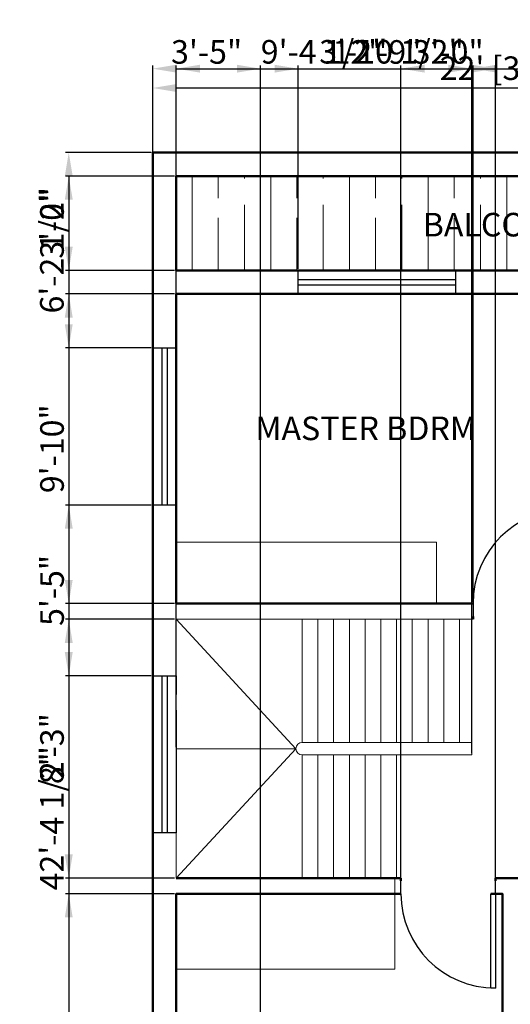
# Model space of a CAD drawing. Units: inches. Extents: x 2429 to 3343, y 1496 to 2530.
# Tile 6 of 7: x 2954 to 3141, y 2154 to 2529. Entities that reach past the tile are written whole.
import ezdxf

# ---------------------------------------------------------------- set-up
doc = ezdxf.new("R2010")
doc.units = ezdxf.units.IN
for name, color, linetype, lineweight in [('A-ANNO-DIMS', 2, 'Continuous', 18), ('A-AREA-IDEN', 3, 'Continuous', 18), ('A-DOOR', 3, 'Continuous', 25), ('A-FLOR-PATT', 8, 'Continuous', 13), ('A-FLOR-STRS', 2, 'Continuous', 18), ('A-FURN', 9, 'Continuous', 18), ('A-GLAZ', 4, 'Continuous', 25), ('A-WALL', 7, 'Continuous', 50)]:
    doc.layers.add(name, color=color, linetype=linetype, lineweight=lineweight)
doc.styles.get("Standard").update_dxf_attribs({"font": 'arial.ttf'})
doc.dimstyles.new('ISO-25', dxfattribs={"dimtxt": 9, "dimasz": 9, "dimexe": 1.25, "dimexo": 0.625, "dimtad": 1, "dimdec": 1, "dimlunit": 3, "dimtxsty": 'Standard', "dimcen": 9, "dimadec": 0, "dimazin": 0, "dimtfac": 1, "dimtdec": 1, "dimtmove": 0, "dimatfit": 3, "dimfxl": 1, "dimarcsym": 0})

# ---------------------------------------------------------------- blocks, each defined once
blk = doc.blocks.new('*D9')
at = {"layer": 'A-ANNO-DIMS', "color": 0, "lineweight": -2, "transparency": 16777216}
for p, q in [((3005.05, 2479.42), (3005.05, 2504.67)), ((3269.05, 2479.42), (3269.05, 2504.67)), ((3014.05, 2503.42), (3260.05, 2503.42))]:
    blk.add_line(p, q, dxfattribs=at)
at = {"layer": 'A-ANNO-DIMS', "color": 0, "transparency": 16777216}
for points in [[(3014.05, 2504.92), (3014.05, 2501.92), (3005.05, 2503.42)], [(3260.05, 2504.92), (3260.05, 2501.92), (3269.05, 2503.42)]]:
    blk.add_solid(points, dxfattribs=at)
at = {"layer": 'Defpoints', "color": 0, "transparency": 16777216}
for p in [(3269.05, 2503.42), (3005.05, 2478.79), (3269.05, 2478.79)]:
    blk.add_point(p, dxfattribs=at)
at = {"layer": 'A-ANNO-DIMS', "color": 0, "transparency": 16777216, "insert": (3137.05, 2509.81), "char_height": 9, "attachment_point": 5}
blk.add_mtext("22' [33']", dxfattribs=at)
blk = doc.blocks.new('*U2')
for p, q in [((0, 0), (0, -5)), ((-36, 0), (-36, -5))]:
    blk.add_line(p, q)
blk.add_lwpolyline([(0, 0), (0, 36), (-1.75, 36), (-1.75, 0)], close=True)
blk.add_arc((0, 0), 36, 90, 180)
blk = doc.blocks.new('*U12')
for p, q in [((-36, 0), (-36, 5)), ((0, 0), (0, 5))]:
    blk.add_line(p, q)
blk.add_lwpolyline([(0, 0), (0, -36), (-1.75, -36), (-1.75, 0)], close=True)
blk.add_arc((0, 0), 36, 180, 270)
blk = doc.blocks.new('WIN-PLAN-1500')
for p, q in [((3.5, 60), (3.5, 0)), ((5.5, 60), (5.5, 0))]:
    blk.add_line(p, q)
blk.add_lwpolyline([(9, 60), (9, 0), (0, 0), (0, 60)], close=True)
blk = doc.blocks.new('*D56')
at = {"layer": 'A-ANNO-DIMS', "color": 0, "lineweight": -2, "transparency": 16777216}
for p, q in [((3004.42, 2478.79), (2971.8, 2478.79)), ((2973.05, 2469.79), (2973.05, 1979.47)), ((3134.79, 1970.47), (2971.8, 1970.47))]:
    blk.add_line(p, q, dxfattribs=at)
at = {"layer": 'A-ANNO-DIMS', "color": 0, "transparency": 16777216}
for points in [[(2971.55, 2469.79), (2974.55, 2469.79), (2973.05, 2478.79)], [(2971.55, 1979.47), (2974.55, 1979.47), (2973.05, 1970.47)]]:
    blk.add_solid(points, dxfattribs=at)
at = {"layer": 'Defpoints', "color": 0, "transparency": 16777216}
for p in [(3005.05, 2478.79), (2973.05, 1970.47), (3135.41, 1970.47)]:
    blk.add_point(p, dxfattribs=at)
at = {"layer": 'A-ANNO-DIMS', "color": 0, "transparency": 16777216, "insert": (2967.77, 2224.63), "char_height": 9, "attachment_point": 5, "rotation": 90}
blk.add_mtext('42\'-4 1/2"', dxfattribs=at)
blk = doc.blocks.new('*D57')
at = {"layer": 'A-ANNO-DIMS', "color": 0, "lineweight": -2, "transparency": 16777216}
for p, q in [((3013.42, 2469.79), (2971.8, 2469.79)), ((2973.05, 2460.79), (2973.05, 2442.79)), ((3013.42, 2433.79), (2971.8, 2433.79))]:
    blk.add_line(p, q, dxfattribs=at)
at = {"layer": 'A-ANNO-DIMS', "color": 0, "transparency": 16777216}
for points in [[(2971.55, 2460.79), (2974.55, 2460.79), (2973.05, 2469.79)], [(2971.55, 2442.79), (2974.55, 2442.79), (2973.05, 2433.79)]]:
    blk.add_solid(points, dxfattribs=at)
at = {"layer": 'Defpoints', "color": 0, "transparency": 16777216}
for p in [(3014.05, 2469.79), (2973.05, 2433.79), (3014.05, 2433.79)]:
    blk.add_point(p, dxfattribs=at)
at = {"layer": 'A-ANNO-DIMS', "color": 0, "transparency": 16777216, "insert": (2967.83, 2451.79), "char_height": 9, "attachment_point": 5, "rotation": 90}
blk.add_mtext('3\'-0"', dxfattribs=at)
blk = doc.blocks.new('*D58')
at = {"layer": 'A-ANNO-DIMS', "color": 0, "lineweight": -2, "transparency": 16777216}
for p, q in [((3014.05, 2425.42), (3014.05, 2512.04)), ((3167.05, 2425.42), (3167.05, 2512.04)), ((3023.05, 2510.79), (3158.05, 2510.79))]:
    blk.add_line(p, q, dxfattribs=at)
at = {"layer": 'A-ANNO-DIMS', "color": 0, "transparency": 16777216}
for points in [[(3023.05, 2512.29), (3023.05, 2509.29), (3014.05, 2510.79)], [(3158.05, 2512.29), (3158.05, 2509.29), (3167.05, 2510.79)]]:
    blk.add_solid(points, dxfattribs=at)
at = {"layer": 'Defpoints', "color": 0, "transparency": 16777216}
for p in [(3167.05, 2510.79), (3014.05, 2424.79), (3167.05, 2424.79)]:
    blk.add_point(p, dxfattribs=at)
at = {"layer": 'A-ANNO-DIMS', "color": 0, "transparency": 16777216, "insert": (3090.55, 2516.01), "char_height": 9, "attachment_point": 5}
blk.add_mtext('12\'-9"', dxfattribs=at)
blk = doc.blocks.new('*D59')
at = {"layer": 'A-ANNO-DIMS', "color": 0, "lineweight": -2, "transparency": 16777216}
for p, q in [((3013.42, 2424.79), (2971.8, 2424.79)), ((2973.05, 2415.79), (2973.05, 2315.58)), ((3013.42, 2306.58), (2971.8, 2306.58))]:
    blk.add_line(p, q, dxfattribs=at)
at = {"layer": 'A-ANNO-DIMS', "color": 0, "transparency": 16777216}
for points in [[(2971.55, 2415.79), (2974.55, 2415.79), (2973.05, 2424.79)], [(2971.55, 2315.58), (2974.55, 2315.58), (2973.05, 2306.58)]]:
    blk.add_solid(points, dxfattribs=at)
at = {"layer": 'Defpoints', "color": 0, "transparency": 16777216}
for p in [(3014.05, 2424.79), (2973.05, 2306.58), (3014.05, 2306.58)]:
    blk.add_point(p, dxfattribs=at)
at = {"layer": 'A-ANNO-DIMS', "color": 0, "transparency": 16777216, "insert": (2967.83, 2365.69), "char_height": 9, "attachment_point": 5, "rotation": 90}
blk.add_mtext('9\'-10"', dxfattribs=at)
blk = doc.blocks.new('*D63')
at = {"layer": 'A-ANNO-DIMS', "color": 0, "lineweight": -2, "transparency": 16777216}
for p, q in [((3013.42, 2300.58), (2971.8, 2300.58)), ((2973.05, 2291.58), (2973.05, 2210.79)), ((3013.42, 2201.79), (2971.8, 2201.79))]:
    blk.add_line(p, q, dxfattribs=at)
at = {"layer": 'A-ANNO-DIMS', "color": 0, "transparency": 16777216}
for points in [[(2971.55, 2291.58), (2974.55, 2291.58), (2973.05, 2300.58)], [(2971.55, 2210.79), (2974.55, 2210.79), (2973.05, 2201.79)]]:
    blk.add_solid(points, dxfattribs=at)
at = {"layer": 'Defpoints', "color": 0, "transparency": 16777216}
for p in [(3014.05, 2300.58), (2973.05, 2201.79), (3014.05, 2201.79)]:
    blk.add_point(p, dxfattribs=at)
at = {"layer": 'A-ANNO-DIMS', "color": 0, "transparency": 16777216, "insert": (2967.83, 2251.18), "char_height": 9, "attachment_point": 5, "rotation": 90}
blk.add_mtext('8\'-3"', dxfattribs=at)
blk = doc.blocks.new('*D64')
at = {"layer": 'A-ANNO-DIMS', "color": 0, "lineweight": -2, "transparency": 16777216}
for p, q in [((3014.05, 2251.81), (3014.05, 2512.04)), ((3126.78, 2249.41), (3126.78, 2512.04)), ((3023.05, 2510.79), (3117.78, 2510.79))]:
    blk.add_line(p, q, dxfattribs=at)
at = {"layer": 'A-ANNO-DIMS', "color": 0, "transparency": 16777216}
for points in [[(3023.05, 2512.29), (3023.05, 2509.29), (3014.05, 2510.79)], [(3117.78, 2512.29), (3117.78, 2509.29), (3126.78, 2510.79)]]:
    blk.add_solid(points, dxfattribs=at)
at = {"layer": 'Defpoints', "color": 0, "transparency": 16777216}
for p in [(3126.78, 2510.79), (3014.05, 2251.18), (3126.78, 2248.78)]:
    blk.add_point(p, dxfattribs=at)
at = {"layer": 'A-ANNO-DIMS', "color": 0, "transparency": 16777216, "insert": (3070.41, 2516.07), "char_height": 9, "attachment_point": 5}
blk.add_mtext('9\'-4 1/2"', dxfattribs=at)
blk = doc.blocks.new('*D66')
at = {"layer": 'A-ANNO-DIMS', "color": 0, "lineweight": -2, "transparency": 16777216}
for p, q in [((3013.42, 2195.79), (2971.8, 2195.79)), ((2973.05, 2186.79), (2973.05, 2036.79)), ((3013.42, 2027.79), (2971.8, 2027.79))]:
    blk.add_line(p, q, dxfattribs=at)
at = {"layer": 'A-ANNO-DIMS', "color": 0, "transparency": 16777216}
for points in [[(2971.55, 2186.79), (2974.55, 2186.79), (2973.05, 2195.79)], [(2971.55, 2036.79), (2974.55, 2036.79), (2973.05, 2027.79)]]:
    blk.add_solid(points, dxfattribs=at)
at = {"layer": 'Defpoints', "color": 0, "transparency": 16777216}
for p in [(3014.05, 2195.79), (2973.05, 2027.79), (3014.05, 2027.79)]:
    blk.add_point(p, dxfattribs=at)
at = {"layer": 'A-ANNO-DIMS', "color": 0, "transparency": 16777216, "insert": (2967.83, 2111.79), "char_height": 9, "attachment_point": 5, "rotation": 90}
blk.add_mtext('14\'-0"', dxfattribs=at)
blk = doc.blocks.new('*D71')
at = {"layer": 'A-ANNO-DIMS', "color": 0, "lineweight": -2, "transparency": 16777216}
for p, q in [((3014.05, 2434.42), (3014.05, 2512.04)), ((3060.55, 2434.42), (3060.55, 2512.04)), ((3023.05, 2510.79), (3051.55, 2510.79)), ((3060.55, 2510.79), (3122.68, 2510.79))]:
    blk.add_line(p, q, dxfattribs=at)
at = {"layer": 'A-ANNO-DIMS', "color": 0, "transparency": 16777216}
for points in [[(3023.05, 2512.29), (3023.05, 2509.29), (3014.05, 2510.79)], [(3051.55, 2512.29), (3051.55, 2509.29), (3060.55, 2510.79)]]:
    blk.add_solid(points, dxfattribs=at)
at = {"layer": 'Defpoints', "color": 0, "transparency": 16777216}
for p in [(3060.55, 2510.79), (3014.05, 2433.79), (3060.55, 2433.79)]:
    blk.add_point(p, dxfattribs=at)
at = {"layer": 'A-ANNO-DIMS', "color": 0, "transparency": 16777216, "insert": (3096.11, 2516.07), "char_height": 9, "attachment_point": 5}
blk.add_mtext('3\'-10 1/2"', dxfattribs=at)
blk = doc.blocks.new('*D72')
at = {"layer": 'A-ANNO-DIMS', "color": 0, "lineweight": -2, "transparency": 16777216}
for p, q in [((3004.42, 2478.79), (2971.8, 2478.79)), ((2973.05, 2469.79), (2973.05, 2413.19)), ((3004.42, 2404.19), (2971.8, 2404.19))]:
    blk.add_line(p, q, dxfattribs=at)
at = {"layer": 'A-ANNO-DIMS', "color": 0, "transparency": 16777216}
for points in [[(2971.55, 2469.79), (2974.55, 2469.79), (2973.05, 2478.79)], [(2971.55, 2413.19), (2974.55, 2413.19), (2973.05, 2404.19)]]:
    blk.add_solid(points, dxfattribs=at)
at = {"layer": 'Defpoints', "color": 0, "transparency": 16777216}
for p in [(3005.05, 2478.79), (2973.05, 2404.19), (3005.05, 2404.19)]:
    blk.add_point(p, dxfattribs=at)
at = {"layer": 'A-ANNO-DIMS', "color": 0, "transparency": 16777216, "insert": (2967.77, 2441.49), "char_height": 9, "attachment_point": 5, "rotation": 90}
blk.add_mtext('6\'-2 1/2"', dxfattribs=at)
blk = doc.blocks.new('*D73')
at = {"layer": 'A-ANNO-DIMS', "color": 0, "lineweight": -2, "transparency": 16777216}
for p, q in [((3004.42, 2344.19), (2971.8, 2344.19)), ((2973.05, 2335.19), (2973.05, 2288.03)), ((3004.42, 2279.03), (2971.8, 2279.03))]:
    blk.add_line(p, q, dxfattribs=at)
at = {"layer": 'A-ANNO-DIMS', "color": 0, "transparency": 16777216}
for points in [[(2971.55, 2335.19), (2974.55, 2335.19), (2973.05, 2344.19)], [(2971.55, 2288.03), (2974.55, 2288.03), (2973.05, 2279.03)]]:
    blk.add_solid(points, dxfattribs=at)
at = {"layer": 'Defpoints', "color": 0, "transparency": 16777216}
for p in [(3005.05, 2344.19), (2973.05, 2279.03), (3005.05, 2279.03)]:
    blk.add_point(p, dxfattribs=at)
at = {"layer": 'A-ANNO-DIMS', "color": 0, "transparency": 16777216, "insert": (2967.85, 2311.61), "char_height": 9, "attachment_point": 5, "rotation": 90}
blk.add_mtext('5\'-5"', dxfattribs=at)
blk = doc.blocks.new('*D76')
at = {"layer": 'A-ANNO-DIMS', "color": 0, "lineweight": -2, "transparency": 16777216}
for p, q in [((3005.05, 2019.41), (3005.05, 2512.04)), ((3046.2, 2019.41), (3046.2, 2512.04)), ((3014.05, 2510.79), (3037.2, 2510.79))]:
    blk.add_line(p, q, dxfattribs=at)
at = {"layer": 'A-ANNO-DIMS', "color": 0, "transparency": 16777216}
for points in [[(3014.05, 2512.29), (3014.05, 2509.29), (3005.05, 2510.79)], [(3037.2, 2512.29), (3037.2, 2509.29), (3046.2, 2510.79)]]:
    blk.add_solid(points, dxfattribs=at)
at = {"layer": 'Defpoints', "color": 0, "transparency": 16777216}
for p in [(3046.2, 2510.79), (3005.05, 2018.79), (3046.2, 2018.79)]:
    blk.add_point(p, dxfattribs=at)
at = {"layer": 'A-ANNO-DIMS', "color": 0, "transparency": 16777216, "insert": (3025.62, 2516.02), "char_height": 9, "attachment_point": 5}
blk.add_mtext('3\'-5"', dxfattribs=at)
blk = doc.blocks.new('*D79')
at = {"layer": 'A-ANNO-DIMS', "color": 0, "lineweight": -2, "transparency": 16777216}
for p, q in [((3127.2, 2307.21), (3127.2, 2512.04)), ((3161.45, 2307.21), (3161.45, 2512.04)), ((3136.2, 2510.79), (3152.45, 2510.79)), ((3161.45, 2510.79), (3223.74, 2510.79))]:
    blk.add_line(p, q, dxfattribs=at)
at = {"layer": 'A-ANNO-DIMS', "color": 0, "transparency": 16777216}
for points in [[(3136.2, 2512.29), (3136.2, 2509.29), (3127.2, 2510.79)], [(3152.45, 2512.29), (3152.45, 2509.29), (3161.45, 2510.79)]]:
    blk.add_solid(points, dxfattribs=at)
at = {"layer": 'Defpoints', "color": 0, "transparency": 16777216}
for p in [(3161.45, 2510.79), (3127.2, 2306.58), (3161.45, 2306.58)]:
    blk.add_point(p, dxfattribs=at)
at = {"layer": 'A-ANNO-DIMS', "color": 0, "transparency": 16777216, "insert": (3197.09, 2516.07), "char_height": 9, "attachment_point": 5}
blk.add_mtext('2\'-10 1/2"', dxfattribs=at)
blk = doc.blocks.new('*D81')
at = {"layer": 'A-ANNO-DIMS', "color": 0, "lineweight": -2, "transparency": 16777216}
for p, q in [((3099.72, 2196.41), (3099.72, 2512.04)), ((3135.72, 2196.41), (3135.72, 2512.04)), ((3108.72, 2510.79), (3126.72, 2510.79))]:
    blk.add_line(p, q, dxfattribs=at)
at = {"layer": 'A-ANNO-DIMS', "color": 0, "transparency": 16777216}
for points in [[(3108.72, 2512.29), (3108.72, 2509.29), (3099.72, 2510.79)], [(3126.72, 2512.29), (3126.72, 2509.29), (3135.72, 2510.79)]]:
    blk.add_solid(points, dxfattribs=at)
at = {"layer": 'Defpoints', "color": 0, "transparency": 16777216}
for p in [(3135.72, 2510.79), (3099.72, 2195.79), (3135.72, 2195.79)]:
    blk.add_point(p, dxfattribs=at)
at = {"layer": 'A-ANNO-DIMS', "color": 0, "transparency": 16777216, "insert": (3117.72, 2516.02), "char_height": 9, "attachment_point": 5}
blk.add_mtext('3\'-0"', dxfattribs=at)

msp = doc.modelspace()

# ---------------------------------------------------------------- hatches: boundary and pattern name
at = {"layer": 'A-FLOR-PATT'}
h = msp.add_hatch(dxfattribs=at)
h.set_pattern_fill('GOST_WOOD', color=256, scale=5)
h.set_pattern_definition([(90, (3260.048, 2433.792), (30, -2e-15), [50, -10]), (90, (3270.048, 2423.792), (30, -2e-15), [30, -7.5, 15, -7.5]), (90, (3280.048, 2408.792), (30, -2e-15), [50, -10])])
h.paths.add_polyline_path([(3260.04839, 2469.7918), (3014.04839, 2469.7918), (3014.04839, 2433.7918), (3260.04839, 2433.7918)])
h.paths.add_polyline_path([(3104.56895, 2440.5916), (3163.9551, 2440.5916), (3163.9551, 2462.39929), (3104.56895, 2462.39929)], flags=24)

# ---------------------------------------------------------------- linework, layer by layer
at = {"layer": 'A-FLOR-STRS'}
for p, q in [((3014.04839, 2300.58253), (3127.19704, 2300.58253)), ((3062.04839, 2300.58253), (3062.04839, 2253.58451)), ((3068.04839, 2300.58253), (3068.04839, 2253.58451)), ((3074.04839, 2300.58253), (3074.04839, 2253.58451)), ((3080.04839, 2300.58253), (3080.04839, 2253.58451)), ((3086.04839, 2300.58253), (3086.04839, 2253.58451)), ((3092.04839, 2300.58253), (3092.04839, 2253.58451)), ((3098.04839, 2300.58253), (3098.04839, 2253.58451)), ((3104.04839, 2300.58253), (3104.04839, 2253.58451)), ((3110.04839, 2300.58253), (3110.04839, 2253.58451)), ((3116.04839, 2300.58253), (3116.04839, 2253.58451)), ((3122.04839, 2300.58253), (3122.04839, 2253.58451)), ((3059.64839, 2251.18451), (3014.04839, 2251.18451)), ((3068.04839, 2248.78451), (3068.04839, 2201.78649)), ((3074.04839, 2248.78451), (3074.04839, 2201.78649)), ((3080.04839, 2248.78451), (3080.04839, 2201.78649)), ((3086.04839, 2248.78451), (3086.04839, 2201.78649)), ((3092.04839, 2248.78451), (3092.04839, 2201.78649)), ((3098.04839, 2248.78451), (3098.04839, 2201.78649))]:
    msp.add_line(p, q, dxfattribs=at)
msp.add_lwpolyline([(3014.04839, 2300.58253), (3059.64839, 2251.18451), (3014.04839, 2201.78649)], close=True, dxfattribs=at)
msp.add_lwpolyline([(3126.78141, 2253.58451), (3126.78141, 2248.78451), (3062.04839, 2248.78451, -1), (3062.04839, 2253.58451)], format="xyb", close=True, dxfattribs=at)
msp.add_lwpolyline([(3062.04839, 2248.78451), (3062.04839, 2246.78451), (3062.04839, 2201.78649)], dxfattribs=at)
at = {"layer": 'A-FURN'}
for points in [[(3014.04839, 2329.96827), (3113.28676, 2329.96827), (3113.28676, 2306.58253)], [(3014.04839, 2167.02265), (3097.44138, 2167.02265), (3097.44138, 2201.78649)]]:
    msp.add_lwpolyline(points, dxfattribs=at)
at = {"layer": 'A-GLAZ'}
for p, q in [((3008.54839, 2279.02781), (3008.54839, 2219.02781)), ((3010.54839, 2279.02781), (3010.54839, 2219.02781))]:
    msp.add_line(p, q, dxfattribs=at)
msp.add_lwpolyline([(3014.04839, 2265.82385), (3014.04839, 2219.02781), (3005.04839, 2219.02781), (3005.04839, 2279.02781), (3014.04839, 2279.02781), (3014.04839, 2271.82385)], dxfattribs=at)
at = {"layer": 'A-WALL'}
for p, q in [((3127.19704, 2301.58253), (3127.19704, 2300.58253)), ((3099.7165, 2200.78649), (3099.7165, 2201.78649)), ((3135.7165, 2200.78649), (3135.7165, 2201.78649))]:
    msp.add_line(p, q, dxfattribs=at)
for points in [[(3135.41055, 1970.47184), (3269.04839, 1970.47184), (3269.04839, 2001.78649), (3269.04839, 2325.78649), (3269.04839, 2478.7918), (3005.04839, 2478.7918), (3005.04839, 2325.78649), (3005.04839, 2319.78649), (3005.04839, 2199.78649), (3005.04839, 2018.78649), (3135.41055, 2018.78649)], [(3260.04839, 2469.7918), (3014.04839, 2469.7918), (3014.04839, 2433.7918), (3260.04839, 2433.7918)]]:
    msp.add_lwpolyline(points, close=True, dxfattribs=at)
for points in [[(3127.19704, 2306.58253), (3014.04839, 2306.58253), (3014.04839, 2319.78649), (3014.04839, 2325.78649), (3014.04839, 2424.7918), (3167.04839, 2424.7918), (3167.04839, 2420.74151)], [(3099.7165, 2201.78649), (3014.04839, 2201.78649)], [(3149.96707, 2201.78649), (3135.7165, 2201.78649)], [(3133.9665, 2195.78649), (3138.41055, 2195.78649), (3138.41055, 2027.78649), (3014.04839, 2027.78649), (3014.04839, 2195.78649), (3099.7165, 2195.78649)]]:
    msp.add_lwpolyline(points, dxfattribs=at)

# ---------------------------------------------------------------- block references
at = {"layer": 'A-DOOR'}
for name, p in [('*U2', (3163.19704, 2306.58253)), ('*U12', (3135.7165, 2195.78649))]:
    msp.add_blockref(name, p, dxfattribs=at)
at = {"layer": 'A-GLAZ', "rotation": 90.0000000000009}
msp.add_blockref('WIN-PLAN-1500', (3120.54875, 2424.79223), dxfattribs=at)
at = {"layer": 'A-GLAZ'}
msp.add_blockref('WIN-PLAN-1500', (3005.04882, 2344.19377), dxfattribs=at)

# ---------------------------------------------------------------- texts
at = {"layer": 'A-AREA-IDEN', "char_height": 9, "attachment_point": 1}
for s, width, insert in [('{\\fCalibri|b0|i0|c0|p34;BALCONY}', 63.8011805, (3108.00972, 2455.73929)), ('{\\fCalibri|b0|i0|c0|p34;MASTER BDRM}', 85.7220201, (3044.19274, 2377.97646))]:
    msp.add_mtext_dynamic_manual_height_columns(s, width=width, gutter_width=12.5, heights=[0], dxfattribs=dict(at, insert=insert))

# ---------------------------------------------------------------- dimensions: what is measured, and where the dimension line sits
at = {"layer": 'A-ANNO-DIMS'}
for base, p1, p2, override, picture, middle in [((3060.54839, 2510.7918), (3014.04839, 2433.7918), (3060.54839, 2433.7918), {"dimdec": 1, "dimlfac": 1, "dimrnd": 0, "dimzin": 1, "dimdsep": 46, "dimlunit": 4, "dimfrac": 2}, '*D71', (3096.11439, 2516.07335)), ((3126.78141, 2510.7918), (3014.04839, 2251.18451), (3126.78141, 2248.78451), {"dimdec": 1, "dimlfac": 1, "dimrnd": 0, "dimzin": 1, "dimdsep": 46, "dimlunit": 4, "dimfrac": 2}, '*D64', (3070.4149, 2516.07028)), ((3161.447043, 2510.791805), (3127.197043, 2306.582531), (3161.447043, 2306.582531), {"dimdec": 1, "dimlfac": 1, "dimrnd": 0, "dimzin": 1, "dimdsep": 46, "dimlunit": 4, "dimfrac": 2}, '*D79', (3197.0928479113, 2516.070283854)), ((3269.04839, 2503.41546), (3005.04839, 2478.7918), (3269.04839, 2478.7918), {"dimclrd": 0, "dimclre": 0, "dimclrt": 0}, '*D9', (3137.04839, 2509.8082)), ((3046.19896, 2510.7918), (3005.04839, 2018.78649), (3046.19896, 2018.78649), {"dimdec": 1, "dimlfac": 1, "dimrnd": 0, "dimzin": 1, "dimdsep": 46, "dimlunit": 4, "dimfrac": 2}, '*D76', (3025.62368, 2516.01503)), ((3167.04839, 2510.7918), (3014.04839, 2424.7918), (3167.04839, 2424.7918), {"dimdec": 1, "dimlfac": 1, "dimrnd": 0, "dimzin": 1, "dimdsep": 46, "dimlunit": 4, "dimfrac": 2}, '*D58', (3090.54839, 2516.01196)), ((3135.7165, 2510.7918), (3099.7165, 2195.78649), (3135.7165, 2195.78649), {"dimdec": 1, "dimlfac": 1, "dimrnd": 0, "dimzin": 1, "dimdsep": 46, "dimlunit": 4, "dimfrac": 2}, '*D81', (3117.7165, 2516.01503))]:
    dim = msp.add_linear_dim(base=base, p1=p1, p2=p2, dimstyle='ISO-25', override=override, dxfattribs=at)
    dim.commit()
    dim.dimension.update_dxf_attribs({"geometry": picture, "text_midpoint": middle})
for base, p1, p2, picture, middle in [((2973.04839, 1970.47184), (3005.04839, 2478.7918), (3135.41055, 1970.47184), '*D56', (2967.76991, 2224.63182)), ((2973.04839, 2404.19413), (3005.04839, 2478.7918), (3005.04839, 2404.19413), '*D72', (2967.76991, 2441.49297)), ((2973.04839, 2433.7918), (3014.04839, 2469.7918), (3014.04839, 2433.7918), '*D57', (2967.82517, 2451.7918)), ((2973.04839, 2306.58253), (3014.04839, 2424.7918), (3014.04839, 2306.58253), '*D59', (2967.82824, 2365.68717)), ((2973.04839, 2279.02781), (3005.04839, 2344.19413), (3005.04839, 2279.02781), '*D73', (2967.84665, 2311.61097)), ((2973.04839, 2201.78649), (3014.04839, 2300.58253), (3014.04839, 2201.78649), '*D63', (2967.82517, 2251.18451)), ((2973.04839, 2027.78649), (3014.04839, 2195.78649), (3014.04839, 2027.78649), '*D66', (2967.82824, 2111.78649))]:
    dim = msp.add_linear_dim(base=base, p1=p1, p2=p2, angle=90, dimstyle='ISO-25', override={"dimdec": 1, "dimlfac": 1, "dimrnd": 0, "dimzin": 1, "dimdsep": 46, "dimlunit": 4, "dimfrac": 2}, dxfattribs=at)
    dim.commit()
    dim.dimension.update_dxf_attribs({"geometry": picture, "text_midpoint": middle})

doc.saveas('drawing.dxf')
